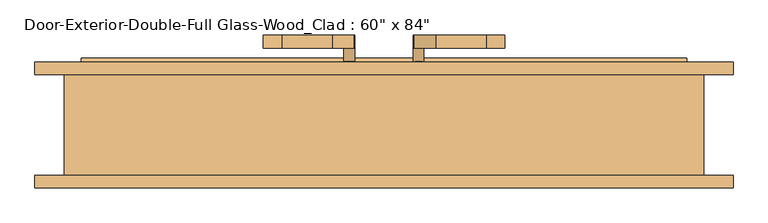
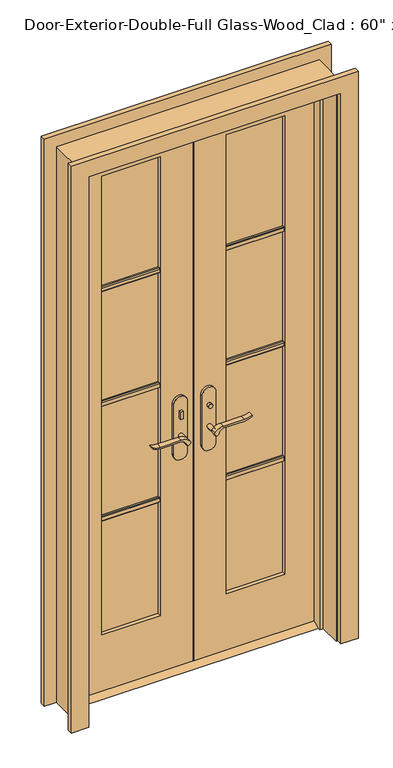
"""IFC4 building model written with IfcOpenShell, lengths in millimetres: door geometry."""

from ifc_helpers import new_model, si_unit, point, frame, frame_2d, origin, place, context, project, spatial, polyline, circle_curve, trimmed, segment, composite_curve, outline, extrude, faceted_brep, source, transform, mapped, element, save


def door_665efd91(model_context):
    return source(origin(), model_context, "Body", "SolidModel", [
        extrude(outline(polyline([(38.1, 12.7), (73.025, 12.7), (98.425, 0.0), (12.7, 0.0), (38.1, 12.7)])), frame((-457.2, 0.0, 0.0), z_axis=(1.0, 0.0, 0.0), x_axis=(0.0, 1.0, 0.0)), (0.0, 0.0, 1.0), 914.4),
        extrude(outline(polyline([(-47.4019111, 18.1), (-57.4019111, 18.1), (-57.4019111, 28.1), (-47.4019111, 28.1), (-47.4019111, 18.1)])), frame((0.0, 0.0, 981.9), z_axis=(0.0, 0.0, 1.0), x_axis=(1.0, 0.0, 0.0)), (0.0, 0.0, 1.0), 30.0),
        extrude(outline(composite_curve([segment(trimmed(circle_curve(frame_2d((996.9, -52.4019111)), 8.0), [point((996.9, -60.4019111))], [point((996.9, -44.4019111))], False, "CARTESIAN"), True, "CONTINUOUS"), segment(trimmed(circle_curve(frame_2d((996.9, -52.4019111)), 8.0), [point((996.9, -44.4019111))], [point((996.9, -60.4019111))], False, "CARTESIAN"), True, "CONTINUOUS")], self_intersect=False)), frame((0.0, 83.025, 0.0), z_axis=(0.0, 1.0, 0.0), x_axis=(0.0, 0.0, 1.0)), (0.0, 0.0, 1.0), 10.0),
        extrude(outline(composite_curve([segment(trimmed(circle_curve(frame_2d((897.1555521, -76.0694241)), 37.2832219), [point((919.0523287, -45.8937749))], [point((934.4, -77.7693445))], False, "CARTESIAN"), True, "CONTINUOUS"), segment(polyline([(934.4, -77.7693445), (934.4, -154.045502)]), True, "CONTINUOUS"), segment(trimmed(circle_curve(frame_2d((1017.6850638, -153.9791202)), 83.2850902), [point((934.4, -154.045502))], [point((939.4, -182.4019111))], True, "CARTESIAN"), True, "CONTINUOUS"), segment(polyline([(939.4, -182.4019111), (936.6135558, -182.4019111)]), True, "CONTINUOUS"), segment(trimmed(circle_curve(frame_2d((986.6709207, -150.4622499)), 59.3791355), [point((936.6135558, -182.4019111))], [point((927.4, -154.045502))], False, "CARTESIAN"), True, "CONTINUOUS"), segment(polyline([(927.4, -154.045502), (927.4, -77.7881013)]), True, "CONTINUOUS"), segment(trimmed(circle_curve(frame_2d((909.2738613, -77.7881013)), 18.1261387), [point((927.4, -77.7881013))], [point((914.4, -60.4019111))], True, "CARTESIAN"), True, "CONTINUOUS"), segment(trimmed(circle_curve(frame_2d((914.4, -52.4019111)), 8.0), [point((914.4, -60.4019111))], [point((919.0523287, -45.8937749))], False, "CARTESIAN"), True, "CONTINUOUS")], self_intersect=False)), frame((0.0, -21.9, 0.0), z_axis=(0.0, 1.0, 0.0), x_axis=(0.0, 0.0, 1.0)), (0.0, 0.0, 1.0), 20.0),
        extrude(outline(composite_curve([segment(trimmed(circle_curve(frame_2d((914.4, -52.4019111)), 8.0), [point((914.3999903, -60.4019111))], [point((919.0523287, -45.8937749))], False, "CARTESIAN"), True, "CONTINUOUS"), segment(trimmed(circle_curve(frame_2d((897.1555521, -76.0694241)), 37.2832219), [point((919.0523287, -45.8937749))], [point((934.4, -77.7693445))], False, "CARTESIAN"), True, "CONTINUOUS"), segment(polyline([(934.4, -77.7693445), (934.4, -154.045502)]), True, "CONTINUOUS"), segment(trimmed(circle_curve(frame_2d((1017.6850638, -153.9791202)), 83.2850902), [point((934.4, -154.045502))], [point((939.4, -182.4019111))], True, "CARTESIAN"), True, "CONTINUOUS"), segment(polyline([(939.4, -182.4019111), (936.6135558, -182.4019111)]), True, "CONTINUOUS"), segment(trimmed(circle_curve(frame_2d((986.6709207, -150.4622499)), 59.3791355), [point((936.6135558, -182.4019111))], [point((927.4, -154.045502))], False, "CARTESIAN"), True, "CONTINUOUS"), segment(polyline([(927.4, -154.045502), (927.4, -77.788099)]), True, "CONTINUOUS"), segment(trimmed(circle_curve(frame_2d((909.2738682, -77.788099)), 18.1261318), [point((927.4, -77.788099))], [point((914.3999903, -60.4019111))], True, "CARTESIAN"), True, "CONTINUOUS")], self_intersect=False)), frame((0.0, 113.025, 0.0), z_axis=(0.0, 1.0, 0.0), x_axis=(0.0, 0.0, 1.0)), (0.0, 0.0, 1.0), 20.0),
        extrude(outline(composite_curve([segment(trimmed(circle_curve(frame_2d((914.4, -52.4019111)), 8.0), [point((914.4, -60.4019111))], [point((914.4, -44.4019111))], False, "CARTESIAN"), True, "CONTINUOUS"), segment(trimmed(circle_curve(frame_2d((914.4, -52.4019111)), 8.0), [point((914.4, -44.4019111))], [point((914.4, -60.4019111))], False, "CARTESIAN"), True, "CONTINUOUS")], self_intersect=False)), frame((0.0, -1.9, 0.0), z_axis=(0.0, 1.0, 0.0), x_axis=(0.0, 0.0, 1.0)), (0.0, 0.0, 1.0), 30.0),
        extrude(outline(composite_curve([segment(trimmed(circle_curve(frame_2d((914.4, -52.4019111)), 8.0), [point((914.4, -60.4019111))], [point((914.4, -44.4019111))], False, "CARTESIAN"), True, "CONTINUOUS"), segment(trimmed(circle_curve(frame_2d((914.4, -52.4019111)), 8.0), [point((914.4, -44.4019111))], [point((914.4, -60.4019111))], False, "CARTESIAN"), True, "CONTINUOUS")], self_intersect=False)), frame((0.0, 83.025, 0.0), z_axis=(0.0, 1.0, 0.0), x_axis=(0.0, 0.0, 1.0)), (0.0, 0.0, 1.0), 30.0),
        extrude(outline(composite_curve([segment(polyline([(844.4, -27.4019111), (1039.4, -27.4019111)]), True, "CONTINUOUS"), segment(trimmed(circle_curve(frame_2d((1039.4, -52.4019111)), 25.0), [point((1039.4, -27.4019111))], [point((1039.4, -77.4019111))], False, "CARTESIAN"), True, "CONTINUOUS"), segment(polyline([(1039.4, -77.4019111), (844.4, -77.4019111)]), True, "CONTINUOUS"), segment(trimmed(circle_curve(frame_2d((844.4, -52.4019111)), 25.0), [point((844.4, -77.4019111))], [point((844.4, -27.4019111))], False, "CARTESIAN"), True, "CONTINUOUS")], self_intersect=False)), frame((0.0, 28.1, 0.0), z_axis=(0.0, 1.0, 0.0), x_axis=(0.0, 0.0, 1.0)), (0.0, 0.0, 1.0), 10.0),
        extrude(outline(composite_curve([segment(polyline([(844.4, -27.4019111), (1039.4, -27.4019111)]), True, "CONTINUOUS"), segment(trimmed(circle_curve(frame_2d((1039.4, -52.4019111)), 25.0), [point((1039.4, -27.4019111))], [point((1039.4, -77.4019111))], False, "CARTESIAN"), True, "CONTINUOUS"), segment(polyline([(1039.4, -77.4019111), (844.4, -77.4019111)]), True, "CONTINUOUS"), segment(trimmed(circle_curve(frame_2d((844.4, -52.4019111)), 25.0), [point((844.4, -77.4019111))], [point((844.4, -27.4019111))], False, "CARTESIAN"), True, "CONTINUOUS")], self_intersect=False)), frame((0.0, 73.025, 0.0), z_axis=(0.0, 1.0, 0.0), x_axis=(0.0, 0.0, 1.0)), (0.0, 0.0, 1.0), 10.0),
        extrude(outline(polyline([(47.3875, 93.025), (57.3875, 93.025), (57.3875, 83.025), (47.3875, 83.025), (47.3875, 93.025)])), frame((0.0, 0.0, 981.9), z_axis=(0.0, 0.0, 1.0), x_axis=(1.0, 0.0, 0.0)), (0.0, 0.0, 1.0), 30.0),
        extrude(outline(composite_curve([segment(trimmed(circle_curve(frame_2d((996.9, 52.3875)), 8.0), [point((996.9, 60.3875))], [point((996.9, 44.3875))], False, "CARTESIAN"), True, "CONTINUOUS"), segment(trimmed(circle_curve(frame_2d((996.9, 52.3875)), 8.0), [point((996.9, 44.3875))], [point((996.9, 60.3875))], False, "CARTESIAN"), True, "CONTINUOUS")], self_intersect=False)), frame((0.0, 18.1, 0.0), z_axis=(0.0, 1.0, 0.0), x_axis=(0.0, 0.0, 1.0)), (0.0, 0.0, 1.0), 10.0),
        extrude(outline(composite_curve([segment(trimmed(circle_curve(frame_2d((914.4, 52.3875)), 8.0), [point((919.0523287, 45.8793637))], [point((914.4, 60.3875))], False, "CARTESIAN"), True, "CONTINUOUS"), segment(trimmed(circle_curve(frame_2d((909.2738613, 77.7736901)), 18.1261387), [point((914.4, 60.3875))], [point((927.4, 77.7736901))], True, "CARTESIAN"), True, "CONTINUOUS"), segment(polyline([(927.4, 77.7736901), (927.4, 154.0310909)]), True, "CONTINUOUS"), segment(trimmed(circle_curve(frame_2d((986.6709207, 150.4478388)), 59.3791355), [point((927.4, 154.0310909))], [point((936.6135558, 182.3875))], False, "CARTESIAN"), True, "CONTINUOUS"), segment(polyline([(936.6135558, 182.3875), (939.4, 182.3875)]), True, "CONTINUOUS"), segment(trimmed(circle_curve(frame_2d((1017.6850638, 153.9647091)), 83.2850902), [point((939.4, 182.3875))], [point((934.4, 154.0310909))], True, "CARTESIAN"), True, "CONTINUOUS"), segment(polyline([(934.4, 154.0310909), (934.4, 77.7549333)]), True, "CONTINUOUS"), segment(trimmed(circle_curve(frame_2d((897.1555521, 76.0550129)), 37.2832219), [point((934.4, 77.7549333))], [point((919.0523287, 45.8793637))], False, "CARTESIAN"), True, "CONTINUOUS")], self_intersect=False)), frame((0.0, 113.025, 0.0), z_axis=(0.0, 1.0, 0.0), x_axis=(0.0, 0.0, 1.0)), (0.0, 0.0, 1.0), 20.0),
        extrude(outline(composite_curve([segment(trimmed(circle_curve(frame_2d((909.2738682, 77.7736878)), 18.1261318), [point((914.3999903, 60.3875))], [point((927.4, 77.7736878))], True, "CARTESIAN"), True, "CONTINUOUS"), segment(polyline([(927.4, 77.7736878), (927.4, 154.0310909)]), True, "CONTINUOUS"), segment(trimmed(circle_curve(frame_2d((986.6709207, 150.4478388)), 59.3791355), [point((927.4, 154.0310909))], [point((936.6135558, 182.3875))], False, "CARTESIAN"), True, "CONTINUOUS"), segment(polyline([(936.6135558, 182.3875), (939.4, 182.3875)]), True, "CONTINUOUS"), segment(trimmed(circle_curve(frame_2d((1017.6850638, 153.9647091)), 83.2850902), [point((939.4, 182.3875))], [point((934.4, 154.0310909))], True, "CARTESIAN"), True, "CONTINUOUS"), segment(polyline([(934.4, 154.0310909), (934.4, 77.7549333)]), True, "CONTINUOUS"), segment(trimmed(circle_curve(frame_2d((897.1555521, 76.0550129)), 37.2832219), [point((934.4, 77.7549333))], [point((919.0523287, 45.8793637))], False, "CARTESIAN"), True, "CONTINUOUS"), segment(trimmed(circle_curve(frame_2d((914.4, 52.3875)), 8.0), [point((919.0523287, 45.8793637))], [point((914.3999903, 60.3875))], False, "CARTESIAN"), True, "CONTINUOUS")], self_intersect=False)), frame((0.0, -21.9, 0.0), z_axis=(0.0, 1.0, 0.0), x_axis=(0.0, 0.0, 1.0)), (0.0, 0.0, 1.0), 20.0),
        extrude(outline(composite_curve([segment(trimmed(circle_curve(frame_2d((914.4, 52.3875)), 8.0), [point((914.4, 60.3875))], [point((914.4, 44.3875))], False, "CARTESIAN"), True, "CONTINUOUS"), segment(trimmed(circle_curve(frame_2d((914.4, 52.3875)), 8.0), [point((914.4, 44.3875))], [point((914.4, 60.3875))], False, "CARTESIAN"), True, "CONTINUOUS")], self_intersect=False)), frame((0.0, 83.025, 0.0), z_axis=(0.0, 1.0, 0.0), x_axis=(0.0, 0.0, 1.0)), (0.0, 0.0, 1.0), 30.0),
        extrude(outline(composite_curve([segment(trimmed(circle_curve(frame_2d((914.4, 52.3875)), 8.0), [point((914.4, 60.3875))], [point((914.4, 44.3875))], False, "CARTESIAN"), True, "CONTINUOUS"), segment(trimmed(circle_curve(frame_2d((914.4, 52.3875)), 8.0), [point((914.4, 44.3875))], [point((914.4, 60.3875))], False, "CARTESIAN"), True, "CONTINUOUS")], self_intersect=False)), frame((0.0, -1.9, 0.0), z_axis=(0.0, 1.0, 0.0), x_axis=(0.0, 0.0, 1.0)), (0.0, 0.0, 1.0), 30.0),
        extrude(outline(composite_curve([segment(trimmed(circle_curve(frame_2d((844.4, 52.3875)), 25.0), [point((844.4, 27.3875))], [point((844.4, 77.3875))], False, "CARTESIAN"), True, "CONTINUOUS"), segment(polyline([(844.4, 77.3875), (1039.4, 77.3875)]), True, "CONTINUOUS"), segment(trimmed(circle_curve(frame_2d((1039.4, 52.3875)), 25.0), [point((1039.4, 77.3875))], [point((1039.4, 27.3875))], False, "CARTESIAN"), True, "CONTINUOUS"), segment(polyline([(1039.4, 27.3875), (844.4, 27.3875)]), True, "CONTINUOUS")], self_intersect=False)), frame((0.0, 73.025, 0.0), z_axis=(0.0, 1.0, 0.0), x_axis=(0.0, 0.0, 1.0)), (0.0, 0.0, 1.0), 10.0),
        extrude(outline(composite_curve([segment(trimmed(circle_curve(frame_2d((844.4, 52.3875)), 25.0), [point((844.4, 27.3875))], [point((844.4, 77.3875))], False, "CARTESIAN"), True, "CONTINUOUS"), segment(polyline([(844.4, 77.3875), (1039.4, 77.3875)]), True, "CONTINUOUS"), segment(trimmed(circle_curve(frame_2d((1039.4, 52.3875)), 25.0), [point((1039.4, 77.3875))], [point((1039.4, 27.3875))], False, "CARTESIAN"), True, "CONTINUOUS"), segment(polyline([(1039.4, 27.3875), (844.4, 27.3875)]), True, "CONTINUOUS")], self_intersect=False)), frame((0.0, 28.1, 0.0), z_axis=(0.0, 1.0, 0.0), x_axis=(0.0, 0.0, 1.0)), (0.0, 0.0, 1.0), 10.0),
        extrude(outline(polyline([(52.07, 1578.371875), (52.07, 1559.321875), (45.72, 1559.321875), (42.545, 1562.496875), (42.545, 1575.196875), (45.72, 1578.371875), (52.07, 1578.371875)])), frame((120.65, 0.0, 0.0), z_axis=(1.0, 0.0, 0.0), x_axis=(0.0, 1.0, 0.0)), (0.0, 0.0, 1.0), 215.9),
        extrude(outline(polyline([(52.07, 1132.68125), (52.07, 1113.63125), (45.72, 1113.63125), (42.545, 1116.80625), (42.545, 1129.50625), (45.72, 1132.68125), (52.07, 1132.68125)])), frame((120.65, 0.0, 0.0), z_axis=(1.0, 0.0, 0.0), x_axis=(0.0, 1.0, 0.0)), (0.0, 0.0, 1.0), 215.9),
        extrude(outline(polyline([(52.07, 686.990625), (52.07, 667.940625), (45.72, 667.940625), (42.545, 671.115625), (42.545, 683.815625), (45.72, 686.990625), (52.07, 686.990625)])), frame((120.65, 0.0, 0.0), z_axis=(1.0, 0.0, 0.0), x_axis=(0.0, 1.0, 0.0)), (0.0, 0.0, 1.0), 215.9),
        extrude(outline(polyline([(59.055, 1578.371875), (65.405, 1578.371875), (68.58, 1575.196875), (68.58, 1562.496875), (65.405, 1559.321875), (59.055, 1559.321875), (59.055, 1578.371875)])), frame((-336.55, 0.0, 0.0), z_axis=(1.0, 0.0, 0.0), x_axis=(0.0, 1.0, 0.0)), (0.0, 0.0, 1.0), 215.9),
        extrude(outline(polyline([(59.055, 1132.68125), (65.405, 1132.68125), (68.58, 1129.50625), (68.58, 1116.80625), (65.405, 1113.63125), (59.055, 1113.63125), (59.055, 1132.68125)])), frame((-336.55, 0.0, 0.0), z_axis=(1.0, 0.0, 0.0), x_axis=(0.0, 1.0, 0.0)), (0.0, 0.0, 1.0), 215.9),
        extrude(outline(polyline([(59.055, 686.990625), (65.405, 686.990625), (68.58, 683.815625), (68.58, 671.115625), (65.405, 667.940625), (59.055, 667.940625), (59.055, 686.990625)])), frame((-336.55, 0.0, 0.0), z_axis=(1.0, 0.0, 0.0), x_axis=(0.0, 1.0, 0.0)), (0.0, 0.0, 1.0), 215.9),
        extrude(outline(polyline([(59.055, 1578.371875), (65.405, 1578.371875), (68.58, 1575.196875), (68.58, 1562.496875), (65.405, 1559.321875), (59.055, 1559.321875), (59.055, 1578.371875)])), frame((120.65, 0.0, 0.0), z_axis=(1.0, 0.0, 0.0), x_axis=(0.0, 1.0, 0.0)), (0.0, 0.0, 1.0), 215.9),
        extrude(outline(polyline([(59.055, 1132.68125), (65.405, 1132.68125), (68.58, 1129.50625), (68.58, 1116.80625), (65.405, 1113.63125), (59.055, 1113.63125), (59.055, 1132.68125)])), frame((120.65, 0.0, 0.0), z_axis=(1.0, 0.0, 0.0), x_axis=(0.0, 1.0, 0.0)), (0.0, 0.0, 1.0), 215.9),
        extrude(outline(polyline([(59.055, 686.990625), (65.405, 686.990625), (68.58, 683.815625), (68.58, 671.115625), (65.405, 667.940625), (59.055, 667.940625), (59.055, 686.990625)])), frame((120.65, 0.0, 0.0), z_axis=(1.0, 0.0, 0.0), x_axis=(0.0, 1.0, 0.0)), (0.0, 0.0, 1.0), 215.9),
        extrude(outline(polyline([(52.07, 1578.371875), (52.07, 1559.321875), (45.72, 1559.321875), (42.545, 1562.496875), (42.545, 1575.196875), (45.72, 1578.371875), (52.07, 1578.371875)])), frame((-336.55, 0.0, 0.0), z_axis=(1.0, 0.0, 0.0), x_axis=(0.0, 1.0, 0.0)), (0.0, 0.0, 1.0), 215.9),
        extrude(outline(polyline([(52.07, 1132.68125), (52.07, 1113.63125), (45.72, 1113.63125), (42.545, 1116.80625), (42.545, 1129.50625), (45.72, 1132.68125), (52.07, 1132.68125)])), frame((-336.55, 0.0, 0.0), z_axis=(1.0, 0.0, 0.0), x_axis=(0.0, 1.0, 0.0)), (0.0, 0.0, 1.0), 215.9),
        extrude(outline(polyline([(52.07, 686.990625), (52.07, 667.940625), (45.72, 667.940625), (42.545, 671.115625), (42.545, 683.815625), (45.72, 686.990625), (52.07, 686.990625)])), frame((-336.55, 0.0, 0.0), z_axis=(1.0, 0.0, 0.0), x_axis=(0.0, 1.0, 0.0)), (0.0, 0.0, 1.0), 215.9),
        extrude(outline(polyline([(0.0, 463.55), (0.0, 527.05), (2203.45, 527.05), (2203.45, -527.05), (0.0, -527.05), (0.0, -463.55), (2139.95, -463.55), (2139.95, 463.55), (0.0, 463.55)])), frame((0.0, 73.025, 0.0), z_axis=(0.0, 1.0, 0.0), x_axis=(0.0, 0.0, 1.0)), (0.0, 0.0, 1.0), 19.05),
        extrude(outline(polyline([(0.0, 463.55), (0.0, 527.05), (2203.45, 527.05), (2203.45, -527.05), (0.0, -527.05), (0.0, -463.55), (2139.95, -463.55), (2139.95, 463.55), (0.0, 463.55)])), frame((0.0, -98.425, 0.0), z_axis=(0.0, 1.0, 0.0), x_axis=(0.0, 0.0, 1.0)), (0.0, 0.0, 1.0), 19.05),
        extrude(outline(polyline([(12.7, 457.2), (2133.6, 457.2), (2133.6, 1.5875), (12.7, 1.5875), (12.7, 457.2)]), holes=[polyline([(2014.5375, 120.65), (2014.5375, 336.55), (231.775, 336.55), (231.775, 120.65), (2014.5375, 120.65)])]), frame((0.0, 38.1, 0.0), z_axis=(0.0, 1.0, 0.0), x_axis=(0.0, 0.0, 1.0)), (0.0, 0.0, 1.0), 34.925),
        extrude(outline(polyline([(2133.6, -457.2), (12.7, -457.2), (12.7, -1.6019111), (2133.6, -1.6019111), (2133.6, -457.2)]), holes=[polyline([(231.775, -336.55), (2014.5375, -336.55), (2014.5375, -120.65), (231.775, -120.65), (231.775, -336.55)])]), frame((0.0, 38.1, 0.0), z_axis=(0.0, 1.0, 0.0), x_axis=(0.0, 0.0, 1.0)), (0.0, 0.0, 1.0), 34.925),
        faceted_brep([(482.6, 73.025, 0.0), (482.6, -79.375, 0.0), (457.2, -79.375, 0.0), (457.2, 3.175, 0.0), (444.5, 3.175, 0.0), (444.5, 38.1, 0.0), (457.2, 38.1, 0.0), (457.2, 73.025, 0.0), (482.6, 73.025, 2159.0), (482.6, -79.375, 2159.0), (-482.6, -79.375, 2159.0), (-482.6, -79.375, 0.0), (-457.2, -79.375, 0.0), (-457.2, -79.375, 2133.6), (457.2, -79.375, 2133.6), (457.2, 3.175, 2133.6), (-457.2, 3.175, 2133.6), (-457.2, 3.175, 0.0), (-444.5, 3.175, 0.0), (-444.5, 3.175, 2120.9), (444.5, 3.175, 2120.9), (444.5, 38.1, 2120.9), (1.5875, 38.1, 2120.9), (-1.6019111, 38.1, 2120.9), (-444.5, 38.1, 2120.9), (-444.5, 38.1, 0.0), (-457.2, 38.1, 0.0), (-457.2, 38.1, 2133.6), (-1.6019111, 38.1, 2133.6), (1.5875, 38.1, 2133.6), (457.2, 38.1, 2133.6), (457.2, 73.025, 2133.6), (1.5875, 73.025, 2133.6), (-1.6019111, 73.025, 2133.6), (-457.2, 73.025, 2133.6), (-457.2, 73.025, 0.0), (-482.6, 73.025, 0.0), (-482.6, 73.025, 2159.0)], [[[0, 1, 2, 3, 4, 5, 6, 7]], [[1, 0, 8, 9]], [[2, 1, 9, 10, 11, 12, 13, 14]], [[3, 2, 14, 15]], [[4, 3, 15, 16, 17, 18, 19, 20]], [[5, 4, 20, 21]], [[6, 5, 21, 22, 23, 24, 25, 26, 27, 28, 29, 30]], [[7, 6, 30, 31]], [[0, 7, 31, 32, 33, 34, 35, 36, 37, 8]], [[9, 8, 37, 10]], [[14, 13, 16, 15]], [[20, 19, 24, 23, 22, 21]], [[31, 30, 29, 28, 27, 34, 33, 32]], [[12, 11, 36, 35, 26, 25, 18, 17]], [[11, 10, 37, 36]], [[13, 12, 17, 16]], [[19, 18, 25, 24]], [[27, 26, 35, 34]]]),
        extrude(outline(polyline([(336.55, 52.07), (120.65, 52.07), (120.65, 59.055), (336.55, 59.055), (336.55, 52.07)])), frame((0.0, 0.0, 231.775), z_axis=(0.0, 0.0, 1.0), x_axis=(1.0, 0.0, 0.0)), (0.0, 0.0, 1.0), 1782.7625),
        extrude(outline(polyline([(-120.65, 52.07), (-336.55, 52.07), (-336.55, 59.055), (-120.65, 59.055), (-120.65, 52.07)])), frame((0.0, 0.0, 231.775), z_axis=(0.0, 0.0, 1.0), x_axis=(1.0, 0.0, 0.0)), (0.0, 0.0, 1.0), 1782.7625),
    ])


if __name__ == "__main__":
    model = new_model("IFC4")
    model_context = context("Model", 3, world=origin())
    ifc_project = project(units=[si_unit("LENGTHUNIT", "METRE", prefix="MILLI")], contexts=[model_context])
    site = spatial("IfcSite", under=ifc_project)
    building = spatial("IfcBuilding", under=site)
    placement = place(None, origin())
    door_shape = door_665efd91(model_context)
    element("IfcDoor", 1, ObjectType="Door-Exterior-Double-Full Glass-Wood_Clad : 60\" x 84\"", at=placement, inside=building, context=model_context, shape_type="MappedRepresentation", body=[
        mapped(door_shape, transform((0.0, 0.0, 0.0), x_axis=(1.0, 0.0, 0.0), y_axis=(0.0, 1.0, 0.0), z_axis=(0.0, 0.0, 1.0))),
    ])
    save(model, "model.ifc")

# Revit data of these elements
# Type "Door-Exterior-Double-Full Glass-Wood_Clad : 60\" x 84\""
#   Type Mark = "8"
#   Assembly Code = "B2030100"
#   Analytic Construction = "French door, wood frame with double glass"
#   Top Rail = 0' - 4 11/16"
#   Threshold Offset [instance default] = 0' - 0 1/2"
#   Thickness = 0' - 1 3/8"
#   Thermal Resistance (R) = 1.9158 (h·ft²·°F)/BTU
#   Swing Angle [instance default] = 90.00°
#   Stiles = 0' - 4 3/4"
#   Rough Width = 3' - 2"
#   Rough Height = 7' - 1"
#   Panel Width = 1' - 6"
#   Door Offset [instance default] = 0' - 0"
#   Height = 7' - 0"
#   Width = 3' - 0"
#   Heat Transfer Coefficient (U) = 0.5220 BTU/(h·ft²·°F)
#   Bottom Rail = 0' - 9 1/8"
#   Exterior Trim [instance default] = yes
#   Threshold [instance default] = yes
#   Show Grill [instance default] = yes
#   Function = 1
#   Trim Material = Cherry
#   Threshold Material = Cherry
#   Panel Material = Cherry
#   Glazing = Glass
#   Frame Material = Cherry
#   Door Handle Material = Aluminum
#   Visual Light Transmittance = 0
#   Solar Heat Gain Coefficient = 0
#   Wall Closure = (empty or 0)
#   Construction Type = (empty or 0)
# Element 1 (IfcDoor, "Door-Exterior-Double-Full Glass-Wood_Clad : 60\" x 84\"")
#   Materials on its faces: "Cherry", "Aluminum", "Glass"
# Materials
#   "Cherry": class "Wood", colour RGB 226 177 128, transparency 0, Description = "Prunus Serotina", Cost = 0
#   "Glass": class "Glass", colour RGB 0 128 192, transparency 0.75, Description = "Soda Lime Glass", Cost = 0
#   "Aluminum": class "Metal", colour RGB 247 247 247, transparency 0, Description = "Aluminum 6061", Cost = 0
